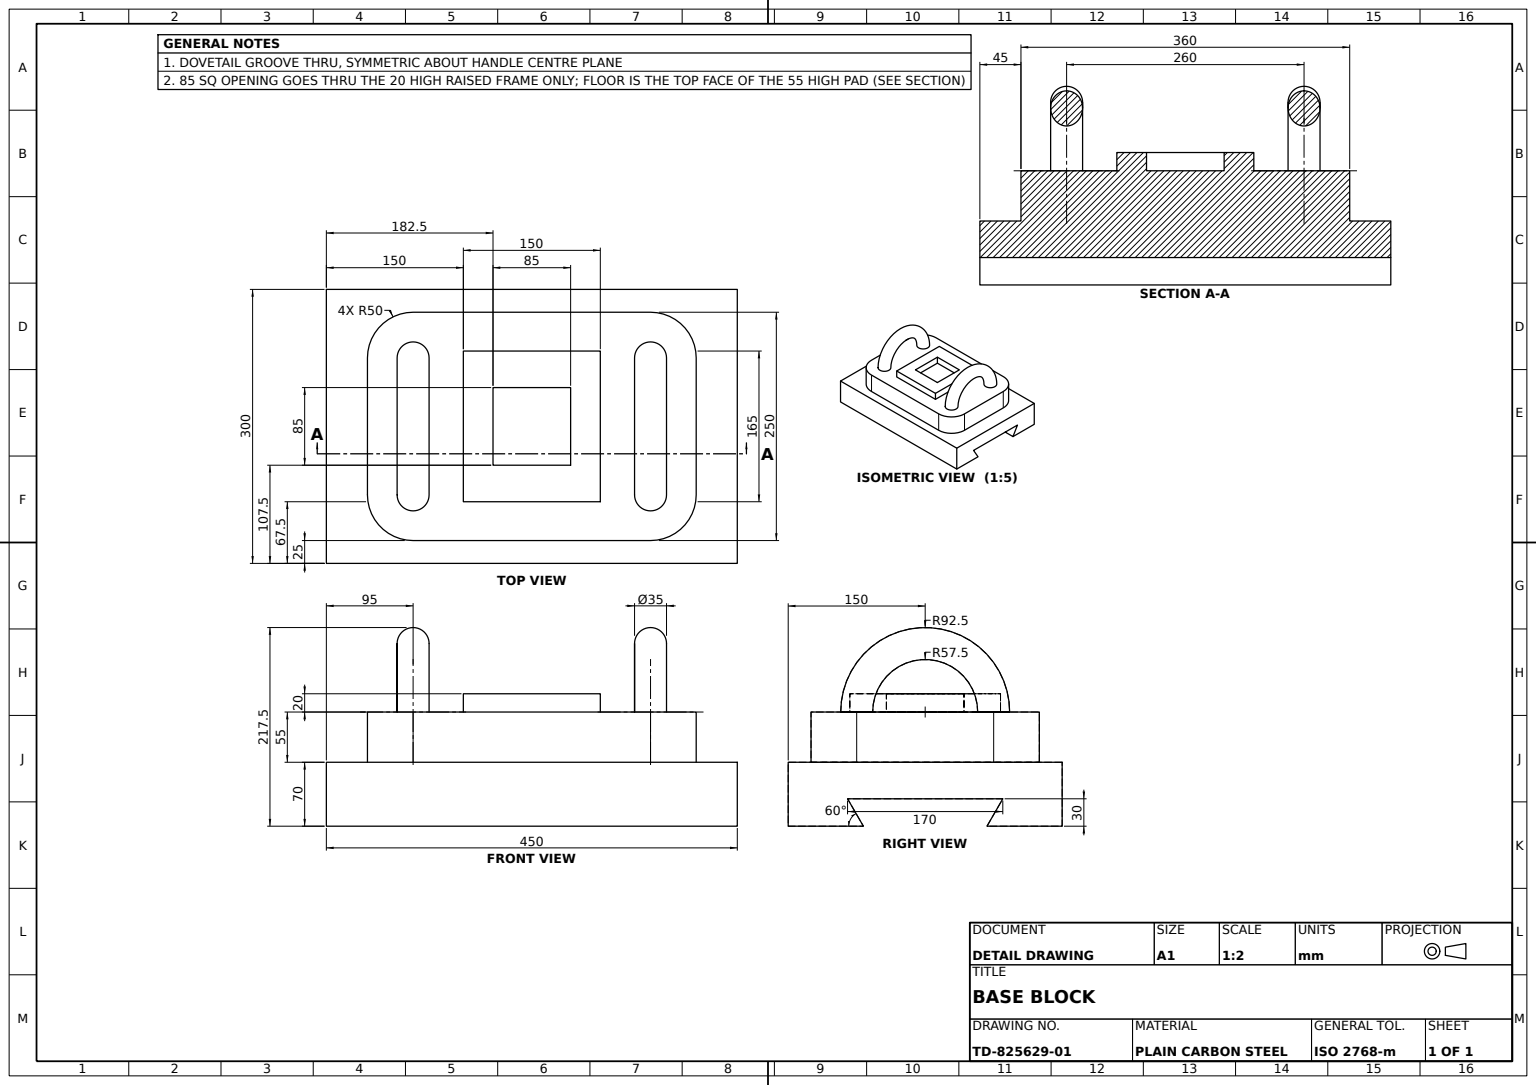
from build123d import *

# Parameters (mm, degrees)
BASE_BLOCK_V_GROOVE_DEPTH   = 225
TOP_PAD_360X250_DEPTH       = 55
SQUARE_FRAME_SKETCH_150_W   = 150
SQUARE_FRAME_SKETCH_150_H   = 165
SQUARE_FRAME_SKETCH_150_W_2 = 85
SQUARE_FRAME_SKETCH_150_H_2 = 85
SQUARE_FRAME_BOSS_150_DEPTH = 20
LIFTING_HANDLE_35_PROFILE_R = 17.5


with BuildPart() as part:
    # Base V-Groove Profile Sketch → Base Block V-Groove (new, symmetric)
    with BuildSketch(Plane(origin=(0, 0, 0), x_dir=(0, 0, -1), z_dir=(1, 0, 0))):
        Polygon((-67.679491924, 0), (-85, 30), (85, 30), (67.679491924, 0), (150, 0), (150, 70), (-150, 70), (-150, 0), align=None)
    extrude(amount=BASE_BLOCK_V_GROOVE_DEPTH, both=True)

    # Top Pad Sketch 360x250 → Top Pad 360x250 (add)
    with BuildSketch(Plane(origin=(0, 70, 0), x_dir=(1, 0, 0), z_dir=(0, 1, 0))):
        with BuildLine():
            Line((-130, -125), (130, -125))
            ThreePointArc((130, -125), (165.355339059, -110.355339059), (180, -75))
            Line((180, -75), (180, 75))
            ThreePointArc((180, 75), (165.355339059, 110.355339059), (130, 125))
            Line((130, 125), (-130, 125))
            ThreePointArc((-130, 125), (-165.355339059, 110.355339059), (-180, 75))
            Line((-180, 75), (-180, -75))
            ThreePointArc((-180, -75), (-165.355339059, -110.355339059), (-130, -125))
        make_face()
    extrude(amount=TOP_PAD_360X250_DEPTH)

    # Square Frame Sketch 150 → Square Frame Boss 150 (add)
    with BuildSketch(Plane(origin=(0, 125, 0), x_dir=(1, 0, 0), z_dir=(0, 1, 0))):
        Rectangle(SQUARE_FRAME_SKETCH_150_W, SQUARE_FRAME_SKETCH_150_H)
        Rectangle(SQUARE_FRAME_SKETCH_150_W_2, SQUARE_FRAME_SKETCH_150_H_2, mode=Mode.SUBTRACT)
    extrude(amount=SQUARE_FRAME_BOSS_150_DEPTH)

    # Lifting Handle Ø35: sweep along a path in Handle Path Sketch
    with BuildLine(Plane(origin=(130, 0, 0), x_dir=(0, 0, -1), z_dir=(1, 0, 0))) as lifting_handle_35_path:
        ThreePointArc((-75, 125), (0, 200), (75, 125))
    # Lifting Handle Ø35 profile (on start of the path) → Lifting Handle Ø35 (sweep)
    with BuildSketch(Plane(origin=(130, 125, 75), x_dir=(0, 0, 1), z_dir=(0, 1, 0))):
        Circle(LIFTING_HANDLE_35_PROFILE_R)
    lifting_handle_35 = sweep(path=lifting_handle_35_path.line)

    # Lifting Handle Mirror: Lifting Handle Ø35 across plane
    add(lifting_handle_35.mirror(Plane(origin=(0, 0, 0), x_dir=(0, 0, 1), z_dir=(1, 0, 0))))


solid = part.part
